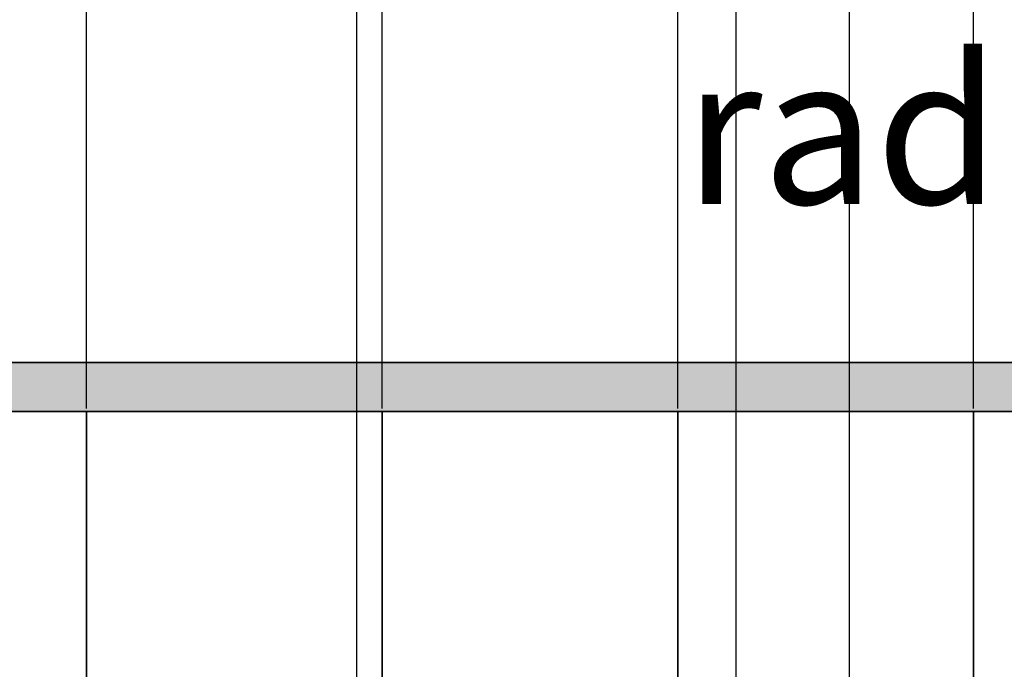
# Model space of a CAD drawing. Units: millimetres. Extents: x -22994 to 29398, y -19990 to 20176.
# Tile 31 of 135: x 119 to 139, y 43 to 56. Entities that reach past the tile are written whole.
import ezdxf

# ---------------------------------------------------------------- set-up
doc = ezdxf.new("R2010")
doc.units = ezdxf.units.MM
doc.header["$MEASUREMENT"] = 0
for name, color, linetype, lineweight in [('M-ANNO-TEXT', 7, 'Continuous', 25), ('M-DIMS', 2, 'Continuous', 18), ('M-EQPM-PATT', 7, 'Continuous', 18), ('M-PIPE', 7, 'Continuous', 35)]:
    doc.layers.add(name, color=color, linetype=linetype, lineweight=lineweight)
doc.styles.get("Standard").update_dxf_attribs({"font": 'arial.ttf'})
doc.dimstyles.get("Standard").update_dxf_attribs({"dimtxt": 0.18, "dimasz": 10000, "dimexe": 0.18, "dimexo": 0.0625, "dimgap": 0.09, "dimtad": 0, "dimtih": 1, "dimtoh": 1, "dimdec": 0, "dimzin": 0, "dimdsep": 46, "dimtxsty": 'Standard', "dimcen": 0.09, "dimadec": 0, "dimazin": 0, "dimtfac": 1, "dimtdec": 0, "dimtofl": 0, "dimtmove": 0, "dimatfit": 3, "dimfxl": 1, "dimtolj": 1, "dimtzin": 0, "dimlwd": 30, "dimarcsym": 0})

# ---------------------------------------------------------------- blocks, each defined once
blk = doc.blocks.new('*D2')
at = {"layer": 'Defpoints', "color": 0, "transparency": 16777216}
for p in [(6.677, 10.271), (290.852, 10.271), (290.852, -5.079)]:
    blk.add_point(p, dxfattribs=at)
at = {"layer": 'M-DIMS', "color": 0, "lineweight": -2, "transparency": 16777216}
for p, q in [((6.677, 10.209), (6.677, -5.259)), ((290.852, 10.209), (290.852, -5.259))]:
    blk.add_line(p, q, dxfattribs=at)
at = {"layer": 'M-DIMS', "color": 0, "lineweight": 30, "transparency": 16777216}
for p, q in [((-9993.323, -5.079), (-19993.323, -5.079)), ((10290.852, -5.079), (20290.852, -5.079))]:
    blk.add_line(p, q, dxfattribs=at)
at = {"layer": 'M-DIMS', "color": 0, "transparency": 16777216}
for points in [[(-9993.323, 1661.588), (-9993.323, -1671.745), (6.677, -5.079)], [(10290.852, 1661.588), (10290.852, -1671.745), (290.852, -5.079)]]:
    blk.add_solid(points, dxfattribs=at)
at = {"layer": 'M-DIMS', "color": 0, "transparency": 16777216, "insert": (148.765, -5.079), "char_height": 0.18, "attachment_point": 5}
blk.add_mtext('\\A1;284.2', dxfattribs=at)
blk = doc.blocks.new('*D3')
at = {"layer": 'Defpoints', "color": 0, "transparency": 16777216}
for p in [(110.265, 204.165), (110.265, 176.366), (95.833, 127.967)]:
    blk.add_point(p, dxfattribs=at)
at = {"layer": 'M-DIMS', "color": 0, "lineweight": -2, "transparency": 16777216}
for p, q in [((95.833, 128.03), (95.833, 204.345)), ((110.265, 176.429), (110.265, 204.345))]:
    blk.add_line(p, q, dxfattribs=at)
at = {"layer": 'M-DIMS', "color": 0, "lineweight": 30, "transparency": 16777216}
for p, q in [((-9904.167, 204.165), (-19904.167, 204.165)), ((10110.265, 204.165), (20110.265, 204.165))]:
    blk.add_line(p, q, dxfattribs=at)
at = {"layer": 'M-DIMS', "color": 0, "transparency": 16777216}
for points in [[(-9904.167, 1870.832), (-9904.167, -1462.501), (95.833, 204.165)], [(10110.265, 1870.832), (10110.265, -1462.501), (110.265, 204.165)]]:
    blk.add_solid(points, dxfattribs=at)
at = {"layer": 'M-DIMS', "color": 0, "transparency": 16777216, "insert": (103.049, 204.165), "char_height": 0.18, "attachment_point": 5}
blk.add_mtext('\\A1;14.432', dxfattribs=at)
blk = doc.blocks.new('*D4')
at = {"layer": 'Defpoints', "color": 0, "transparency": 16777216}
for p in [(116.265, 204.165), (110.265, 176.366), (116.265, 176.366)]:
    blk.add_point(p, dxfattribs=at)
at = {"layer": 'M-DIMS', "color": 0, "lineweight": -2, "transparency": 16777216}
for p, q in [((110.265, 176.429), (110.265, 204.345)), ((116.265, 176.429), (116.265, 204.345))]:
    blk.add_line(p, q, dxfattribs=at)
at = {"layer": 'M-DIMS', "color": 0, "lineweight": 30, "transparency": 16777216}
for p, q in [((-9889.735, 204.165), (-19889.735, 204.165)), ((10116.265, 204.165), (20116.265, 204.165))]:
    blk.add_line(p, q, dxfattribs=at)
at = {"layer": 'M-DIMS', "color": 0, "transparency": 16777216}
for points in [[(-9889.735, 1870.832), (-9889.735, -1462.501), (110.265, 204.165)], [(10116.265, 1870.832), (10116.265, -1462.501), (116.265, 204.165)]]:
    blk.add_solid(points, dxfattribs=at)
at = {"layer": 'M-DIMS', "color": 0, "transparency": 16777216, "insert": (113.265, 204.165), "char_height": 0.18, "attachment_point": 5}
blk.add_mtext('\\A1;6', dxfattribs=at)
blk = doc.blocks.new('*D5')
at = {"layer": 'Defpoints', "color": 0, "transparency": 16777216}
for p in [(181.265, 204.165), (116.265, 176.366), (181.265, 176.366)]:
    blk.add_point(p, dxfattribs=at)
at = {"layer": 'M-DIMS', "color": 0, "lineweight": -2, "transparency": 16777216}
for p, q in [((116.265, 176.429), (116.265, 204.345)), ((181.265, 176.429), (181.265, 204.345))]:
    blk.add_line(p, q, dxfattribs=at)
at = {"layer": 'M-DIMS', "color": 0, "lineweight": 30, "transparency": 16777216}
for p, q in [((-9883.735, 204.165), (-19883.735, 204.165)), ((10181.265, 204.165), (20181.265, 204.165))]:
    blk.add_line(p, q, dxfattribs=at)
at = {"layer": 'M-DIMS', "color": 0, "transparency": 16777216}
for points in [[(-9883.735, 1870.832), (-9883.735, -1462.501), (116.265, 204.165)], [(10181.265, 1870.832), (10181.265, -1462.501), (181.265, 204.165)]]:
    blk.add_solid(points, dxfattribs=at)
at = {"layer": 'M-DIMS', "color": 0, "transparency": 16777216, "insert": (148.765, 204.165), "char_height": 0.18, "attachment_point": 5}
blk.add_mtext('\\A1;65', dxfattribs=at)
blk = doc.blocks.new('*D6')
at = {"layer": 'Defpoints', "color": 0, "transparency": 16777216}
for p in [(187.265, 204.165), (181.265, 176.366), (187.265, 176.366)]:
    blk.add_point(p, dxfattribs=at)
at = {"layer": 'M-DIMS', "color": 0, "lineweight": -2, "transparency": 16777216}
for p, q in [((181.265, 176.429), (181.265, 204.345)), ((187.265, 176.429), (187.265, 204.345))]:
    blk.add_line(p, q, dxfattribs=at)
at = {"layer": 'M-DIMS', "color": 0, "lineweight": 30, "transparency": 16777216}
for p, q in [((-9818.735, 204.165), (-19818.735, 204.165)), ((10187.265, 204.165), (20187.265, 204.165))]:
    blk.add_line(p, q, dxfattribs=at)
at = {"layer": 'M-DIMS', "color": 0, "transparency": 16777216}
for points in [[(-9818.735, 1870.832), (-9818.735, -1462.501), (181.265, 204.165)], [(10187.265, 1870.832), (10187.265, -1462.501), (187.265, 204.165)]]:
    blk.add_solid(points, dxfattribs=at)
at = {"layer": 'M-DIMS', "color": 0, "transparency": 16777216, "insert": (184.265, 204.165), "char_height": 0.18, "attachment_point": 5}
blk.add_mtext('\\A1;6', dxfattribs=at)
blk = doc.blocks.new('*D7')
at = {"layer": 'Defpoints', "color": 0, "transparency": 16777216}
for p in [(201.697, 204.165), (187.265, 176.366), (201.697, 127.967)]:
    blk.add_point(p, dxfattribs=at)
at = {"layer": 'M-DIMS', "color": 0, "lineweight": -2, "transparency": 16777216}
for p, q in [((187.265, 176.429), (187.265, 204.345)), ((201.697, 128.03), (201.697, 204.345))]:
    blk.add_line(p, q, dxfattribs=at)
at = {"layer": 'M-DIMS', "color": 0, "lineweight": 30, "transparency": 16777216}
for p, q in [((-9812.735, 204.165), (-19812.735, 204.165)), ((10201.697, 204.165), (20201.697, 204.165))]:
    blk.add_line(p, q, dxfattribs=at)
at = {"layer": 'M-DIMS', "color": 0, "transparency": 16777216}
for points in [[(-9812.735, 1870.832), (-9812.735, -1462.501), (187.265, 204.165)], [(10201.697, 1870.832), (10201.697, -1462.501), (201.697, 204.165)]]:
    blk.add_solid(points, dxfattribs=at)
at = {"layer": 'M-DIMS', "color": 0, "transparency": 16777216, "insert": (194.481, 204.165), "char_height": 0.18, "attachment_point": 5}
blk.add_mtext('\\A1;14.432', dxfattribs=at)
blk = doc.blocks.new('*D8')
at = {"layer": 'Defpoints', "color": 0, "transparency": 16777216}
for p in [(227.648, 204.165), (227.648, 146.73), (201.697, 127.967)]:
    blk.add_point(p, dxfattribs=at)
at = {"layer": 'M-DIMS', "color": 0, "lineweight": -2, "transparency": 16777216}
for p, q in [((201.697, 128.03), (201.697, 204.345)), ((227.648, 146.792), (227.648, 204.345))]:
    blk.add_line(p, q, dxfattribs=at)
at = {"layer": 'M-DIMS', "color": 0, "lineweight": 30, "transparency": 16777216}
for p, q in [((-9798.303, 204.165), (-19798.303, 204.165)), ((10227.648, 204.165), (20227.648, 204.165))]:
    blk.add_line(p, q, dxfattribs=at)
at = {"layer": 'M-DIMS', "color": 0, "transparency": 16777216}
for points in [[(-9798.303, 1870.832), (-9798.303, -1462.501), (201.697, 204.165)], [(10227.648, 1870.832), (10227.648, -1462.501), (227.648, 204.165)]]:
    blk.add_solid(points, dxfattribs=at)
at = {"layer": 'M-DIMS', "color": 0, "transparency": 16777216, "insert": (214.673, 204.165), "char_height": 0.18, "attachment_point": 5}
blk.add_mtext('\\A1;25.95', dxfattribs=at)
blk = doc.blocks.new('*D9')
at = {"layer": 'Defpoints', "color": 0, "transparency": 16777216}
for p in [(187.265, 176.366), (306.202, 176.366), (290.852, 10.271)]:
    blk.add_point(p, dxfattribs=at)
at = {"layer": 'M-DIMS', "color": 0, "lineweight": 30, "transparency": 16777216}
for p, q in [((306.202, 10176.366), (306.202, 20176.366)), ((306.202, -9989.729), (306.202, -19989.729))]:
    blk.add_line(p, q, dxfattribs=at)
at = {"layer": 'M-DIMS', "color": 0, "lineweight": -2, "transparency": 16777216}
for p, q in [((187.327, 176.366), (306.382, 176.366)), ((290.915, 10.271), (306.382, 10.271))]:
    blk.add_line(p, q, dxfattribs=at)
at = {"layer": 'M-DIMS', "color": 0, "transparency": 16777216}
for points in [[(-1360.465, 10176.366), (1972.869, 10176.366), (306.202, 176.366)], [(-1360.465, -9989.729), (1972.869, -9989.729), (306.202, 10.271)]]:
    blk.add_solid(points, dxfattribs=at)
at = {"layer": 'M-DIMS', "color": 0, "transparency": 16777216, "insert": (306.202, 93.319), "char_height": 0.18, "attachment_point": 5}
blk.add_mtext('\\A1;166.1', dxfattribs=at)
blk = doc.blocks.new('*D10')
at = {"layer": 'Defpoints', "color": 0, "transparency": 16777216}
for p in [(125.65, 136.071), (133.346, 136.071), (133.346, -5.079)]:
    blk.add_point(p, dxfattribs=at)
at = {"layer": 'M-DIMS', "color": 0, "lineweight": -2, "transparency": 16777216}
for p, q in [((125.65, 136.009), (125.65, -5.259)), ((133.346, 136.009), (133.346, -5.259))]:
    blk.add_line(p, q, dxfattribs=at)
at = {"layer": 'M-DIMS', "color": 0, "lineweight": 30, "transparency": 16777216}
for p, q in [((-9874.35, -5.079), (-19874.35, -5.079)), ((10133.346, -5.079), (20133.346, -5.079))]:
    blk.add_line(p, q, dxfattribs=at)
at = {"layer": 'M-DIMS', "color": 0, "transparency": 16777216}
for points in [[(-9874.35, 1661.588), (-9874.35, -1671.745), (125.65, -5.079)], [(10133.346, 1661.588), (10133.346, -1671.745), (133.346, -5.079)]]:
    blk.add_solid(points, dxfattribs=at)
at = {"layer": 'M-DIMS', "color": 0, "transparency": 16777216, "insert": (129.498, -5.079), "char_height": 0.18, "attachment_point": 5}
blk.add_mtext('\\A1;7.696', dxfattribs=at)
blk = doc.blocks.new('*D11')
at = {"layer": 'Defpoints', "color": 0, "transparency": 16777216}
for p in [(133.346, 136.071), (135.65, 136.071), (135.65, -5.079)]:
    blk.add_point(p, dxfattribs=at)
at = {"layer": 'M-DIMS', "color": 0, "lineweight": -2, "transparency": 16777216}
for p, q in [((133.346, 136.009), (133.346, -5.259)), ((135.65, 136.009), (135.65, -5.259))]:
    blk.add_line(p, q, dxfattribs=at)
at = {"layer": 'M-DIMS', "color": 0, "lineweight": 30, "transparency": 16777216}
for p, q in [((-9866.654, -5.079), (-19866.654, -5.079)), ((10135.65, -5.079), (20135.65, -5.079))]:
    blk.add_line(p, q, dxfattribs=at)
at = {"layer": 'M-DIMS', "color": 0, "transparency": 16777216}
for points in [[(-9866.654, 1661.588), (-9866.654, -1671.745), (133.346, -5.079)], [(10135.65, 1661.588), (10135.65, -1671.745), (135.65, -5.079)]]:
    blk.add_solid(points, dxfattribs=at)
at = {"layer": 'M-DIMS', "color": 0, "transparency": 16777216, "insert": (134.498, -5.079), "char_height": 0.18, "attachment_point": 5}
blk.add_mtext('\\A1;2.304', dxfattribs=at)
blk = doc.blocks.new('*D12')
at = {"layer": 'Defpoints', "color": 0, "transparency": 16777216}
for p in [(135.65, 136.071), (145.65, 136.071), (145.65, -5.079)]:
    blk.add_point(p, dxfattribs=at)
at = {"layer": 'M-DIMS', "color": 0, "lineweight": -2, "transparency": 16777216}
for p, q in [((135.65, 136.009), (135.65, -5.259)), ((145.65, 136.009), (145.65, -5.259))]:
    blk.add_line(p, q, dxfattribs=at)
at = {"layer": 'M-DIMS', "color": 0, "lineweight": 30, "transparency": 16777216}
for p, q in [((-9864.35, -5.079), (-19864.35, -5.079)), ((10145.65, -5.079), (20145.65, -5.079))]:
    blk.add_line(p, q, dxfattribs=at)
at = {"layer": 'M-DIMS', "color": 0, "transparency": 16777216}
for points in [[(-9864.35, 1661.588), (-9864.35, -1671.745), (135.65, -5.079)], [(10145.65, 1661.588), (10145.65, -1671.745), (145.65, -5.079)]]:
    blk.add_solid(points, dxfattribs=at)
at = {"layer": 'M-DIMS', "color": 0, "transparency": 16777216, "insert": (140.65, -5.079), "char_height": 0.18, "attachment_point": 5}
blk.add_mtext('\\A1;10', dxfattribs=at)
blk = doc.blocks.new('*D13')
at = {"layer": 'Defpoints', "color": 0, "transparency": 16777216}
for p in [(145.65, 136.071), (155.65, 136.071), (155.65, -5.079)]:
    blk.add_point(p, dxfattribs=at)
at = {"layer": 'M-DIMS', "color": 0, "lineweight": -2, "transparency": 16777216}
for p, q in [((145.65, 136.009), (145.65, -5.259)), ((155.65, 136.009), (155.65, -5.259))]:
    blk.add_line(p, q, dxfattribs=at)
at = {"layer": 'M-DIMS', "color": 0, "lineweight": 30, "transparency": 16777216}
for p, q in [((-9854.35, -5.079), (-19854.35, -5.079)), ((10155.65, -5.079), (20155.65, -5.079))]:
    blk.add_line(p, q, dxfattribs=at)
at = {"layer": 'M-DIMS', "color": 0, "transparency": 16777216}
for points in [[(-9854.35, 1661.588), (-9854.35, -1671.745), (145.65, -5.079)], [(10155.65, 1661.588), (10155.65, -1671.745), (155.65, -5.079)]]:
    blk.add_solid(points, dxfattribs=at)
at = {"layer": 'M-DIMS', "color": 0, "transparency": 16777216, "insert": (150.65, -5.079), "char_height": 0.18, "attachment_point": 5}
blk.add_mtext('\\A1;10', dxfattribs=at)
blk = doc.blocks.new('*D14')
at = {"layer": 'Defpoints', "color": 0, "transparency": 16777216}
for p in [(155.65, 136.071), (165.65, 136.071), (165.65, -5.079)]:
    blk.add_point(p, dxfattribs=at)
at = {"layer": 'M-DIMS', "color": 0, "lineweight": -2, "transparency": 16777216}
for p, q in [((155.65, 136.009), (155.65, -5.259)), ((165.65, 136.009), (165.65, -5.259))]:
    blk.add_line(p, q, dxfattribs=at)
at = {"layer": 'M-DIMS', "color": 0, "lineweight": 30, "transparency": 16777216}
for p, q in [((-9844.35, -5.079), (-19844.35, -5.079)), ((10165.65, -5.079), (20165.65, -5.079))]:
    blk.add_line(p, q, dxfattribs=at)
at = {"layer": 'M-DIMS', "color": 0, "transparency": 16777216}
for points in [[(-9844.35, 1661.588), (-9844.35, -1671.745), (155.65, -5.079)], [(10165.65, 1661.588), (10165.65, -1671.745), (165.65, -5.079)]]:
    blk.add_solid(points, dxfattribs=at)
at = {"layer": 'M-DIMS', "color": 0, "transparency": 16777216, "insert": (160.65, -5.079), "char_height": 0.18, "attachment_point": 5}
blk.add_mtext('\\A1;10', dxfattribs=at)
blk = doc.blocks.new('*D15')
at = {"layer": 'Defpoints', "color": 0, "transparency": 16777216}
for p in [(173.346, 154.788), (173.346, 136.071), (306.202, 136.071)]:
    blk.add_point(p, dxfattribs=at)
at = {"layer": 'M-DIMS', "color": 0, "lineweight": 30, "transparency": 16777216}
for p, q in [((306.202, 10154.788), (306.202, 20154.788)), ((306.202, -9863.929), (306.202, -19863.929))]:
    blk.add_line(p, q, dxfattribs=at)
at = {"layer": 'M-DIMS', "color": 0, "lineweight": -2, "transparency": 16777216}
for p, q in [((173.408, 154.788), (306.382, 154.788)), ((173.408, 136.071), (306.382, 136.071))]:
    blk.add_line(p, q, dxfattribs=at)
at = {"layer": 'M-DIMS', "color": 0, "transparency": 16777216}
for points in [[(-1360.465, 10154.788), (1972.869, 10154.788), (306.202, 154.788)], [(-1360.465, -9863.929), (1972.869, -9863.929), (306.202, 136.071)]]:
    blk.add_solid(points, dxfattribs=at)
at = {"layer": 'M-DIMS', "color": 0, "transparency": 16777216, "insert": (306.202, 145.43), "char_height": 0.18, "attachment_point": 5}
blk.add_mtext('\\A1;18.717', dxfattribs=at)
blk = doc.blocks.new('*D16')
at = {"layer": 'Defpoints', "color": 0, "transparency": 16777216}
for p in [(120.17, 204.165), (110.466, 48.035), (120.17, 48.035)]:
    blk.add_point(p, dxfattribs=at)
at = {"layer": 'M-DIMS', "color": 0, "lineweight": -2, "transparency": 16777216}
for p, q in [((110.466, 48.097), (110.466, 204.345)), ((120.17, 48.097), (120.17, 204.345))]:
    blk.add_line(p, q, dxfattribs=at)
at = {"layer": 'M-DIMS', "color": 0, "lineweight": 30, "transparency": 16777216}
for p, q in [((-9889.534, 204.165), (-19889.534, 204.165)), ((10120.17, 204.165), (20120.17, 204.165))]:
    blk.add_line(p, q, dxfattribs=at)
at = {"layer": 'M-DIMS', "color": 0, "transparency": 16777216}
for points in [[(-9889.534, 1870.832), (-9889.534, -1462.501), (110.466, 204.165)], [(10120.17, 1870.832), (10120.17, -1462.501), (120.17, 204.165)]]:
    blk.add_solid(points, dxfattribs=at)
at = {"layer": 'M-DIMS', "color": 0, "transparency": 16777216, "insert": (115.318, 204.165), "char_height": 0.18, "attachment_point": 5}
blk.add_mtext('\\A1;9.704', dxfattribs=at)
blk = doc.blocks.new('*D17')
at = {"layer": 'Defpoints', "color": 0, "transparency": 16777216}
for p in [(126.17, 204.165), (120.17, 48.035), (126.17, 48.035)]:
    blk.add_point(p, dxfattribs=at)
at = {"layer": 'M-DIMS', "color": 0, "lineweight": -2, "transparency": 16777216}
for p, q in [((120.17, 48.097), (120.17, 204.345)), ((126.17, 48.097), (126.17, 204.345))]:
    blk.add_line(p, q, dxfattribs=at)
at = {"layer": 'M-DIMS', "color": 0, "lineweight": 30, "transparency": 16777216}
for p, q in [((-9879.83, 204.165), (-19879.83, 204.165)), ((10126.17, 204.165), (20126.17, 204.165))]:
    blk.add_line(p, q, dxfattribs=at)
at = {"layer": 'M-DIMS', "color": 0, "transparency": 16777216}
for points in [[(-9879.83, 1870.832), (-9879.83, -1462.501), (120.17, 204.165)], [(10126.17, 1870.832), (10126.17, -1462.501), (126.17, 204.165)]]:
    blk.add_solid(points, dxfattribs=at)
at = {"layer": 'M-DIMS', "color": 0, "transparency": 16777216, "insert": (123.17, 204.165), "char_height": 0.18, "attachment_point": 5}
blk.add_mtext('\\A1;6', dxfattribs=at)
blk = doc.blocks.new('*D18')
at = {"layer": 'Defpoints', "color": 0, "transparency": 16777216}
for p in [(132.17, 204.165), (126.17, 48.035), (132.17, 48.035)]:
    blk.add_point(p, dxfattribs=at)
at = {"layer": 'M-DIMS', "color": 0, "lineweight": -2, "transparency": 16777216}
for p, q in [((126.17, 48.097), (126.17, 204.345)), ((132.17, 48.097), (132.17, 204.345))]:
    blk.add_line(p, q, dxfattribs=at)
at = {"layer": 'M-DIMS', "color": 0, "lineweight": 30, "transparency": 16777216}
for p, q in [((-9873.83, 204.165), (-19873.83, 204.165)), ((10132.17, 204.165), (20132.17, 204.165))]:
    blk.add_line(p, q, dxfattribs=at)
at = {"layer": 'M-DIMS', "color": 0, "transparency": 16777216}
for points in [[(-9873.83, 1870.832), (-9873.83, -1462.501), (126.17, 204.165)], [(10132.17, 1870.832), (10132.17, -1462.501), (132.17, 204.165)]]:
    blk.add_solid(points, dxfattribs=at)
at = {"layer": 'M-DIMS', "color": 0, "transparency": 16777216, "insert": (129.17, 204.165), "char_height": 0.18, "attachment_point": 5}
blk.add_mtext('\\A1;6', dxfattribs=at)
blk = doc.blocks.new('*D19')
at = {"layer": 'Defpoints', "color": 0, "transparency": 16777216}
for p in [(138.17, 204.165), (132.17, 48.035), (138.17, 48.035)]:
    blk.add_point(p, dxfattribs=at)
at = {"layer": 'M-DIMS', "color": 0, "lineweight": -2, "transparency": 16777216}
for p, q in [((132.17, 48.097), (132.17, 204.345)), ((138.17, 48.097), (138.17, 204.345))]:
    blk.add_line(p, q, dxfattribs=at)
at = {"layer": 'M-DIMS', "color": 0, "lineweight": 30, "transparency": 16777216}
for p, q in [((-9867.83, 204.165), (-19867.83, 204.165)), ((10138.17, 204.165), (20138.17, 204.165))]:
    blk.add_line(p, q, dxfattribs=at)
at = {"layer": 'M-DIMS', "color": 0, "transparency": 16777216}
for points in [[(-9867.83, 1870.832), (-9867.83, -1462.501), (132.17, 204.165)], [(10138.17, 1870.832), (10138.17, -1462.501), (138.17, 204.165)]]:
    blk.add_solid(points, dxfattribs=at)
at = {"layer": 'M-DIMS', "color": 0, "transparency": 16777216, "insert": (135.17, 204.165), "char_height": 0.18, "attachment_point": 5}
blk.add_mtext('\\A1;6', dxfattribs=at)
blk = doc.blocks.new('*D20')
at = {"layer": 'Defpoints', "color": 0, "transparency": 16777216}
for p in [(144.17, 204.165), (138.17, 48.035), (144.17, 48.035)]:
    blk.add_point(p, dxfattribs=at)
at = {"layer": 'M-DIMS', "color": 0, "lineweight": -2, "transparency": 16777216}
for p, q in [((138.17, 48.097), (138.17, 204.345)), ((144.17, 48.097), (144.17, 204.345))]:
    blk.add_line(p, q, dxfattribs=at)
at = {"layer": 'M-DIMS', "color": 0, "lineweight": 30, "transparency": 16777216}
for p, q in [((-9861.83, 204.165), (-19861.83, 204.165)), ((10144.17, 204.165), (20144.17, 204.165))]:
    blk.add_line(p, q, dxfattribs=at)
at = {"layer": 'M-DIMS', "color": 0, "transparency": 16777216}
for points in [[(-9861.83, 1870.832), (-9861.83, -1462.501), (138.17, 204.165)], [(10144.17, 1870.832), (10144.17, -1462.501), (144.17, 204.165)]]:
    blk.add_solid(points, dxfattribs=at)
at = {"layer": 'M-DIMS', "color": 0, "transparency": 16777216, "insert": (141.17, 204.165), "char_height": 0.18, "attachment_point": 5}
blk.add_mtext('\\A1;6', dxfattribs=at)
blk = doc.blocks.new('*D21')
at = {"layer": 'Defpoints', "color": 0, "transparency": 16777216}
for p in [(149.116, 204.165), (144.17, 48.035), (149.116, 48.035)]:
    blk.add_point(p, dxfattribs=at)
at = {"layer": 'M-DIMS', "color": 0, "lineweight": -2, "transparency": 16777216}
for p, q in [((144.17, 48.097), (144.17, 204.345)), ((149.116, 48.097), (149.116, 204.345))]:
    blk.add_line(p, q, dxfattribs=at)
at = {"layer": 'M-DIMS', "color": 0, "lineweight": 30, "transparency": 16777216}
for p, q in [((-9855.83, 204.165), (-19855.83, 204.165)), ((10149.116, 204.165), (20149.116, 204.165))]:
    blk.add_line(p, q, dxfattribs=at)
at = {"layer": 'M-DIMS', "color": 0, "transparency": 16777216}
for points in [[(-9855.83, 1870.832), (-9855.83, -1462.501), (144.17, 204.165)], [(10149.116, 1870.832), (10149.116, -1462.501), (149.116, 204.165)]]:
    blk.add_solid(points, dxfattribs=at)
at = {"layer": 'M-DIMS', "color": 0, "transparency": 16777216, "insert": (146.643, 204.165), "char_height": 0.18, "attachment_point": 5}
blk.add_mtext('\\A1;4.945', dxfattribs=at)
blk = doc.blocks.new('*D22')
at = {"layer": 'Defpoints', "color": 0, "transparency": 16777216}
for p in [(149.116, 30.99), (155.116, 30.99), (155.116, -5.079)]:
    blk.add_point(p, dxfattribs=at)
at = {"layer": 'M-DIMS', "color": 0, "lineweight": -2, "transparency": 16777216}
for p, q in [((149.116, 30.927), (149.116, -5.259)), ((155.116, 30.927), (155.116, -5.259))]:
    blk.add_line(p, q, dxfattribs=at)
at = {"layer": 'M-DIMS', "color": 0, "lineweight": 30, "transparency": 16777216}
for p, q in [((-9850.884, -5.079), (-19850.884, -5.079)), ((10155.116, -5.079), (20155.116, -5.079))]:
    blk.add_line(p, q, dxfattribs=at)
at = {"layer": 'M-DIMS', "color": 0, "transparency": 16777216}
for points in [[(-9850.884, 1661.588), (-9850.884, -1671.745), (149.116, -5.079)], [(10155.116, 1661.588), (10155.116, -1671.745), (155.116, -5.079)]]:
    blk.add_solid(points, dxfattribs=at)
at = {"layer": 'M-DIMS', "color": 0, "transparency": 16777216, "insert": (152.116, -5.079), "char_height": 0.18, "attachment_point": 5}
blk.add_mtext('\\A1;6', dxfattribs=at)
blk = doc.blocks.new('*D23')
at = {"layer": 'Defpoints', "color": 0, "transparency": 16777216}
for p in [(155.116, 30.99), (161.116, 30.99), (161.116, -5.079)]:
    blk.add_point(p, dxfattribs=at)
at = {"layer": 'M-DIMS', "color": 0, "lineweight": -2, "transparency": 16777216}
for p, q in [((155.116, 30.927), (155.116, -5.259)), ((161.116, 30.927), (161.116, -5.259))]:
    blk.add_line(p, q, dxfattribs=at)
at = {"layer": 'M-DIMS', "color": 0, "lineweight": 30, "transparency": 16777216}
for p, q in [((-9844.884, -5.079), (-19844.884, -5.079)), ((10161.116, -5.079), (20161.116, -5.079))]:
    blk.add_line(p, q, dxfattribs=at)
at = {"layer": 'M-DIMS', "color": 0, "transparency": 16777216}
for points in [[(-9844.884, 1661.588), (-9844.884, -1671.745), (155.116, -5.079)], [(10161.116, 1661.588), (10161.116, -1671.745), (161.116, -5.079)]]:
    blk.add_solid(points, dxfattribs=at)
at = {"layer": 'M-DIMS', "color": 0, "transparency": 16777216, "insert": (158.116, -5.079), "char_height": 0.18, "attachment_point": 5}
blk.add_mtext('\\A1;6', dxfattribs=at)
blk = doc.blocks.new('*D24')
at = {"layer": 'Defpoints', "color": 0, "transparency": 16777216}
for p in [(161.116, 30.99), (166.439, 30.99), (166.439, -5.079)]:
    blk.add_point(p, dxfattribs=at)
at = {"layer": 'M-DIMS', "color": 0, "lineweight": -2, "transparency": 16777216}
for p, q in [((161.116, 30.927), (161.116, -5.259)), ((166.439, 30.927), (166.439, -5.259))]:
    blk.add_line(p, q, dxfattribs=at)
at = {"layer": 'M-DIMS', "color": 0, "lineweight": 30, "transparency": 16777216}
for p, q in [((-9838.884, -5.079), (-19838.884, -5.079)), ((10166.439, -5.079), (20166.439, -5.079))]:
    blk.add_line(p, q, dxfattribs=at)
at = {"layer": 'M-DIMS', "color": 0, "transparency": 16777216}
for points in [[(-9838.884, 1661.588), (-9838.884, -1671.745), (161.116, -5.079)], [(10166.439, 1661.588), (10166.439, -1671.745), (166.439, -5.079)]]:
    blk.add_solid(points, dxfattribs=at)
at = {"layer": 'M-DIMS', "color": 0, "transparency": 16777216, "insert": (163.777, -5.079), "char_height": 0.18, "attachment_point": 5}
blk.add_mtext('\\A1;5.323', dxfattribs=at)
blk = doc.blocks.new('*D25')
at = {"layer": 'Defpoints', "color": 0, "transparency": 16777216}
for p in [(166.439, 30.99), (172.439, 30.99), (172.439, -5.079)]:
    blk.add_point(p, dxfattribs=at)
at = {"layer": 'M-DIMS', "color": 0, "lineweight": -2, "transparency": 16777216}
for p, q in [((166.439, 30.927), (166.439, -5.259)), ((172.439, 30.927), (172.439, -5.259))]:
    blk.add_line(p, q, dxfattribs=at)
at = {"layer": 'M-DIMS', "color": 0, "lineweight": 30, "transparency": 16777216}
for p, q in [((-9833.561, -5.079), (-19833.561, -5.079)), ((10172.439, -5.079), (20172.439, -5.079))]:
    blk.add_line(p, q, dxfattribs=at)
at = {"layer": 'M-DIMS', "color": 0, "transparency": 16777216}
for points in [[(-9833.561, 1661.588), (-9833.561, -1671.745), (166.439, -5.079)], [(10172.439, 1661.588), (10172.439, -1671.745), (172.439, -5.079)]]:
    blk.add_solid(points, dxfattribs=at)
at = {"layer": 'M-DIMS', "color": 0, "transparency": 16777216, "insert": (169.439, -5.079), "char_height": 0.18, "attachment_point": 5}
blk.add_mtext('\\A1;6', dxfattribs=at)
blk = doc.blocks.new('*D26')
at = {"layer": 'Defpoints', "color": 0, "transparency": 16777216}
for p in [(172.439, 30.99), (178.439, 30.99), (178.439, -5.079)]:
    blk.add_point(p, dxfattribs=at)
at = {"layer": 'M-DIMS', "color": 0, "lineweight": -2, "transparency": 16777216}
for p, q in [((172.439, 30.927), (172.439, -5.259)), ((178.439, 30.927), (178.439, -5.259))]:
    blk.add_line(p, q, dxfattribs=at)
at = {"layer": 'M-DIMS', "color": 0, "lineweight": 30, "transparency": 16777216}
for p, q in [((-9827.561, -5.079), (-19827.561, -5.079)), ((10178.439, -5.079), (20178.439, -5.079))]:
    blk.add_line(p, q, dxfattribs=at)
at = {"layer": 'M-DIMS', "color": 0, "transparency": 16777216}
for points in [[(-9827.561, 1661.588), (-9827.561, -1671.745), (172.439, -5.079)], [(10178.439, 1661.588), (10178.439, -1671.745), (178.439, -5.079)]]:
    blk.add_solid(points, dxfattribs=at)
at = {"layer": 'M-DIMS', "color": 0, "transparency": 16777216, "insert": (175.439, -5.079), "char_height": 0.18, "attachment_point": 5}
blk.add_mtext('\\A1;6', dxfattribs=at)
blk = doc.blocks.new('*D27')
at = {"layer": 'Defpoints', "color": 0, "transparency": 16777216}
for p in [(178.439, 30.99), (188.117, 30.99), (188.117, -5.079)]:
    blk.add_point(p, dxfattribs=at)
at = {"layer": 'M-DIMS', "color": 0, "lineweight": -2, "transparency": 16777216}
for p, q in [((178.439, 30.927), (178.439, -5.259)), ((188.117, 30.927), (188.117, -5.259))]:
    blk.add_line(p, q, dxfattribs=at)
at = {"layer": 'M-DIMS', "color": 0, "lineweight": 30, "transparency": 16777216}
for p, q in [((-9821.561, -5.079), (-19821.561, -5.079)), ((10188.117, -5.079), (20188.117, -5.079))]:
    blk.add_line(p, q, dxfattribs=at)
at = {"layer": 'M-DIMS', "color": 0, "transparency": 16777216}
for points in [[(-9821.561, 1661.588), (-9821.561, -1671.745), (178.439, -5.079)], [(10188.117, 1661.588), (10188.117, -1671.745), (188.117, -5.079)]]:
    blk.add_solid(points, dxfattribs=at)
at = {"layer": 'M-DIMS', "color": 0, "transparency": 16777216, "insert": (183.278, -5.079), "char_height": 0.18, "attachment_point": 5}
blk.add_mtext('\\A1;9.679', dxfattribs=at)
blk = doc.blocks.new('*D28')
at = {"layer": 'Defpoints', "color": 0, "transparency": 16777216}
for p in [(188.117, 48.035), (306.202, 48.035), (188.117, 30.99)]:
    blk.add_point(p, dxfattribs=at)
at = {"layer": 'M-DIMS', "color": 0, "lineweight": 30, "transparency": 16777216}
for p, q in [((306.202, 10048.035), (306.202, 20048.035)), ((306.202, -9969.01), (306.202, -19969.01))]:
    blk.add_line(p, q, dxfattribs=at)
at = {"layer": 'M-DIMS', "color": 0, "lineweight": -2, "transparency": 16777216}
for p, q in [((188.18, 48.035), (306.382, 48.035)), ((188.18, 30.99), (306.382, 30.99))]:
    blk.add_line(p, q, dxfattribs=at)
at = {"layer": 'M-DIMS', "color": 0, "transparency": 16777216}
for points in [[(-1360.465, 10048.035), (1972.869, 10048.035), (306.202, 48.035)], [(-1360.465, -9969.01), (1972.869, -9969.01), (306.202, 30.99)]]:
    blk.add_solid(points, dxfattribs=at)
at = {"layer": 'M-DIMS', "color": 0, "transparency": 16777216, "insert": (306.202, 39.512), "char_height": 0.18, "attachment_point": 5}
blk.add_mtext('\\A1;17.045', dxfattribs=at)
blk = doc.blocks.new('*D29')
at = {"layer": 'Defpoints', "color": 0, "transparency": 16777216}
for p in [(36.801, 80.045), (64.03, 80.045)]:
    blk.add_point(p, dxfattribs=at)
at = {"layer": 'M-DIMS', "color": 0, "lineweight": -2, "transparency": 16777216}
for p, q in [((50.415, 79.955), (50.415, 80.135)), ((50.325, 80.045), (50.505, 80.045))]:
    blk.add_line(p, q, dxfattribs=at)
at = {"layer": 'M-DIMS', "color": 0, "lineweight": 30, "transparency": 16777216}
blk.add_line((20064.03, 80.03), (10064.03, 80.038), dxfattribs=at)
at = {"layer": 'M-DIMS', "color": 0, "transparency": 16777216}
blk.add_solid([(10064.031, 1746.704), (10064.028, -1586.629), (64.03, 80.045)], dxfattribs=at)
at = {"layer": 'M-DIMS', "color": 0, "transparency": 16777216, "insert": (20064.521, 80.03), "char_height": 0.18, "attachment_point": 5}
blk.add_mtext('\\A1;∅27.23', dxfattribs=at)
blk = doc.blocks.new('*D36')
at = {"layer": 'Defpoints', "color": 0, "transparency": 16777216}
for p in [(46.39, 31.303), (46.387, 26.593)]:
    blk.add_point(p, dxfattribs=at)
at = {"layer": 'M-DIMS', "color": 0, "lineweight": 30, "transparency": 16777216}
for p, q in [((57.15, 20031.301), (51.77, 10031.302)), ((10057.15, 20031.301), (57.15, 20031.301))]:
    blk.add_line(p, q, dxfattribs=at)
at = {"layer": 'M-DIMS', "color": 0, "lineweight": -2, "transparency": 16777216}
for p, q in [((46.389, 28.858), (46.389, 29.038)), ((46.299, 28.948), (46.479, 28.948))]:
    blk.add_line(p, q, dxfattribs=at)
at = {"layer": 'M-DIMS', "color": 0, "transparency": 16777216}
blk.add_solid([(-1614.896, 10032.199), (1718.436, 10030.405), (46.39, 31.303)], dxfattribs=at)
at = {"layer": 'M-DIMS', "color": 0, "transparency": 16777216, "insert": (10057.554, 20031.301), "char_height": 0.18, "attachment_point": 5}
blk.add_mtext('\\A1;∅4.71', dxfattribs=at)
blk = doc.blocks.new('*D37')
at = {"layer": 'Defpoints', "color": 0, "transparency": 16777216}
for p in [(54.834, 118.615), (59.494, 118.614)]:
    blk.add_point(p, dxfattribs=at)
at = {"layer": 'M-DIMS', "color": 0, "lineweight": -2, "transparency": 16777216}
for p, q in [((57.164, 118.524), (57.164, 118.704)), ((57.074, 118.614), (57.254, 118.614))]:
    blk.add_line(p, q, dxfattribs=at)
at = {"layer": 'M-DIMS', "color": 0, "lineweight": 30, "transparency": 16777216}
blk.add_line((20059.493, 116.253), (10059.494, 117.434), dxfattribs=at)
at = {"layer": 'M-DIMS', "color": 0, "transparency": 16777216}
blk.add_solid([(10059.69, 1784.1), (10059.297, -1549.233), (59.494, 118.614)], dxfattribs=at)
at = {"layer": 'M-DIMS', "color": 0, "transparency": 16777216, "insert": (20059.985, 116.253), "char_height": 0.18, "attachment_point": 5}
blk.add_mtext('\\A1;∅4.659', dxfattribs=at)

msp = doc.modelspace()

# ---------------------------------------------------------------- hatches: boundary and pattern name
at = {"layer": 'M-EQPM-PATT'}
h = msp.add_hatch(color=256, dxfattribs=at)
h.set_gradient(color1=(19, 155, 72), color2=(88, 186, 72), tint=1, name='CYLINDER')
h.paths.add_polyline_path([(109.4658, 29.9895), (189.1175, 29.9895), (189.1175, 77.6953), (128.1172, 77.6953, 0.4142136), (126.1172, 75.6953), (126.1172, 73.6953, 0.4142136), (128.1172, 71.6953), (178.5136, 71.6953, -0.4142136), (179.5136, 70.6953), (179.5136, 68.6953, -0.4142136), (178.5136, 67.6953), (128.1172, 67.6953, 0.4142136), (126.1172, 65.6953), (126.1172, 63.6953, 0.4142136), (128.1172, 61.6953), (178.5136, 61.6953, -0.4142136), (179.5136, 60.6953), (179.5136, 58.6953, -0.4142136), (178.5136, 57.6953), (109.7466, 57.6953, -0.4142136), (108.7466, 58.6953), (108.7466, 75.5922, 0.4142136), (106.7466, 77.5922), (101.8327, 77.5922), (101.8327, 76.5922), (106.7466, 76.5922, -0.4142136), (107.7466, 75.5922), (107.7466, 58.6953, 0.4142136), (109.7466, 56.6953), (178.5136, 56.6953, 0.4142136), (180.5136, 58.6953), (180.5136, 60.6953, 0.4142136), (178.5136, 62.6953), (128.1172, 62.6953, -0.4142136), (127.1172, 63.6953), (127.1172, 65.6953, -0.4142136), (128.1172, 66.6953), (178.5136, 66.6953, 0.4142136), (180.5136, 68.6953), (180.5136, 70.6953, 0.4142136), (178.5136, 72.6953), (128.1172, 72.6953, -0.4142136), (127.1172, 73.6953), (127.1172, 75.6953, -0.4142136), (128.1172, 76.6953), (188.1175, 76.6953), (188.1175, 49.0349), (110.4658, 49.0349), (110.4658, 51.9576), (101.8327, 51.9576), (101.8327, 50.9576), (109.4658, 50.9576), (109.4658, 48.5349)])
h.paths.add_polyline_path([(110.4658, 48.0349), (188.1175, 48.0349), (188.1175, 30.9895), (110.4658, 30.9895)], flags=16)
h.paths.add_polyline_path([(136.1519, 78.0082), (161.2406, 78.0082), (161.2406, 84.1903), (136.1519, 84.1903)], flags=9)

# ---------------------------------------------------------------- linework, layer by layer
at = {"layer": 'M-PIPE'}
for p, q in [((120.1702, 48.0349), (120.1702, 30.9895)), ((126.1702, 48.0349), (126.1702, 30.9895)), ((126.1702, 48.0349), (126.1702, 30.9895)), ((132.1702, 48.0349), (132.1702, 30.9895)), ((132.1702, 48.0349), (132.1702, 30.9895)), ((132.1702, 48.0349), (132.1702, 30.9895)), ((138.1702, 48.0349), (138.1702, 30.9895)), ((138.1702, 48.0349), (138.1702, 30.9895))]:
    msp.add_line(p, q, dxfattribs=at)
for points in [[(110.4658, 49.0349), (188.1175, 49.0349)], [(188.1175, 30.9895), (110.4658, 30.9895), (110.4658, 48.0349), (188.1175, 48.0349)]]:
    msp.add_lwpolyline(points, dxfattribs=at)

# ---------------------------------------------------------------- texts
at = {"layer": 'M-ANNO-TEXT', "insert": (132.2925, 55.25), "char_height": 3, "attachment_point": 1}
msp.add_mtext_dynamic_manual_height_columns('radiant evaporator', width=37.883315, gutter_width=1, heights=[0], dxfattribs=at)

# ---------------------------------------------------------------- dimensions: what is measured, and where the dimension line sits
at = {"layer": 'M-DIMS'}
for base, p1, p2, override, picture, middle in [((306.202, 176.3662), (290.852, 10.2713), (187.2647, 176.3662), {"dimdec": 1, "dimlfac": 1, "dimrnd": 0, "dimzin": 0, "dimdsep": 46, "dimlunit": 2}, '*D9', (306.202, 93.3187)), ((306.202, 136.0713), (173.3459, 154.788), (173.3459, 136.0713), {"dimdec": 3, "dimlfac": 1, "dimrnd": 0, "dimzin": 0, "dimdsep": 46, "dimlunit": 2}, '*D15', (306.202, 145.4297)), ((306.202, 48.0349), (188.1175, 30.9895), (188.1175, 48.0349), {"dimdec": 3, "dimlfac": 1, "dimrnd": 0, "dimzin": 0, "dimdsep": 46, "dimlunit": 2}, '*D28', (306.202, 39.5122))]:
    dim = msp.add_linear_dim(base=base, p1=p1, p2=p2, angle=90, dimstyle='Standard', override=override, dxfattribs=at)
    dim.commit()
    dim.dimension.update_dxf_attribs({"geometry": picture, "text_midpoint": middle})
dim = msp.add_diameter_dim_2p(p1=(46.3875, 26.5934), p2=(46.39, 31.3035), dimstyle='Standard', override={"dimdec": 2, "dimlfac": 1, "dimrnd": 0, "dimzin": 0, "dimdsep": 46, "dimlunit": 2}, dxfattribs=at)
dim.commit()
dim.dimension.update_dxf_attribs({"geometry": '*D36', "text_midpoint": (10057.5542, 20031.3006), "dimtype": 163})
for base, p1, p2, override, picture, middle in [((110.2647, 204.1654), (95.8327, 127.967), (110.2647, 176.3662), {"dimdec": 3, "dimlfac": 1, "dimrnd": 0, "dimzin": 0, "dimdsep": 46, "dimlunit": 2}, '*D3', (103.0487, 204.1654)), ((116.2647, 204.1654), (110.2647, 176.3662), (116.2647, 176.3662), {"dimdec": 0, "dimlfac": 1, "dimrnd": 0, "dimzin": 0, "dimdsep": 46, "dimlunit": 2}, '*D4', (113.2647, 204.1654)), ((120.1702, 204.1654), (110.4658, 48.0349), (120.1702, 48.0349), {"dimdec": 3, "dimlfac": 1, "dimrnd": 0, "dimzin": 0, "dimdsep": 46, "dimlunit": 2}, '*D16', (115.318, 204.1654)), ((181.2647, 204.1654), (116.2647, 176.3662), (181.2647, 176.3662), {"dimdec": 0, "dimlfac": 1, "dimrnd": 0, "dimzin": 0, "dimdsep": 46, "dimlunit": 2}, '*D5', (148.7647, 204.1654)), ((126.1702, 204.1654), (120.1702, 48.0349), (126.1702, 48.0349), {"dimdec": 0, "dimlfac": 1, "dimrnd": 0, "dimzin": 0, "dimdsep": 46, "dimlunit": 2}, '*D17', (123.1702, 204.1654)), ((132.1702, 204.1654), (126.1702, 48.0349), (132.1702, 48.0349), {"dimdec": 0, "dimlfac": 1, "dimrnd": 0, "dimzin": 0, "dimdsep": 46, "dimlunit": 2}, '*D18', (129.1702, 204.1654)), ((138.1702, 204.1654), (132.1702, 48.0349), (138.1702, 48.0349), {"dimdec": 0, "dimlfac": 1, "dimrnd": 0, "dimzin": 0, "dimdsep": 46, "dimlunit": 2}, '*D19', (135.1702, 204.1654)), ((144.1702, 204.1654), (138.1702, 48.0349), (144.1702, 48.0349), {"dimdec": 0, "dimlfac": 1, "dimrnd": 0, "dimzin": 0, "dimdsep": 46, "dimlunit": 2}, '*D20', (141.1702, 204.1654)), ((149.11567, 204.16539), (144.17023, 48.03494), (149.11567, 48.03494), {"dimdec": 3, "dimlfac": 1, "dimrnd": 0, "dimzin": 0, "dimdsep": 46, "dimlunit": 2}, '*D21', (146.64295, 204.16539)), ((187.2647, 204.1654), (181.2647, 176.3662), (187.2647, 176.3662), {"dimdec": 0, "dimlfac": 1, "dimrnd": 0, "dimzin": 0, "dimdsep": 46, "dimlunit": 2}, '*D6', (184.2647, 204.1654)), ((201.6967, 204.1654), (187.2647, 176.3662), (201.6967, 127.967), {"dimdec": 3, "dimlfac": 1, "dimrnd": 0, "dimzin": 0, "dimdsep": 46, "dimlunit": 2}, '*D7', (194.4807, 204.1654)), ((227.6485, 204.1654), (201.6967, 127.967), (227.6485, 146.7296), {"dimdec": 2, "dimlfac": 1, "dimrnd": 0, "dimzin": 0, "dimdsep": 46, "dimlunit": 2}, '*D8', (214.6726, 204.1654)), ((290.852, -5.0787), (6.6773, 10.2713), (290.852, 10.2713), {"dimdec": 1, "dimlfac": 1, "dimrnd": 0, "dimzin": 0, "dimdsep": 46, "dimlunit": 2}, '*D2', (148.7647, -5.0787)), ((133.3459, -5.0787), (125.6498, 136.0713), (133.3459, 136.0713), {"dimdec": 3, "dimlfac": 1, "dimrnd": 0, "dimzin": 0, "dimdsep": 46, "dimlunit": 2}, '*D10', (129.4978, -5.0787)), ((135.6498, -5.0787), (133.3459, 136.0713), (135.6498, 136.0713), {"dimdec": 3, "dimlfac": 1, "dimrnd": 0, "dimzin": 0, "dimdsep": 46, "dimlunit": 2}, '*D11', (134.4978, -5.0787)), ((145.6498, -5.0787), (135.6498, 136.0713), (145.6498, 136.0713), {"dimdec": 0, "dimlfac": 1, "dimrnd": 0, "dimzin": 0, "dimdsep": 46, "dimlunit": 2}, '*D12', (140.6498, -5.0787)), ((155.6498, -5.0787), (145.6498, 136.0713), (155.6498, 136.0713), {"dimdec": 0, "dimlfac": 1, "dimrnd": 0, "dimzin": 0, "dimdsep": 46, "dimlunit": 2}, '*D13', (150.6498, -5.0787)), ((155.1157, -5.0787), (149.1157, 30.9895), (155.1157, 30.9895), {"dimdec": 0, "dimlfac": 1, "dimrnd": 0, "dimzin": 0, "dimdsep": 46, "dimlunit": 2}, '*D22', (152.1157, -5.0787)), ((161.1157, -5.0787), (155.1157, 30.9895), (161.1157, 30.9895), {"dimdec": 0, "dimlfac": 1, "dimrnd": 0, "dimzin": 0, "dimdsep": 46, "dimlunit": 2}, '*D23', (158.1157, -5.0787)), ((165.6498, -5.0787), (155.6498, 136.0713), (165.6498, 136.0713), {"dimdec": 0, "dimlfac": 1, "dimrnd": 0, "dimzin": 0, "dimdsep": 46, "dimlunit": 2}, '*D14', (160.6498, -5.0787)), ((166.4387, -5.0787), (161.1157, 30.9895), (166.4387, 30.9895), {"dimdec": 3, "dimlfac": 1, "dimrnd": 0, "dimzin": 0, "dimdsep": 46, "dimlunit": 2}, '*D24', (163.7772, -5.0787)), ((172.4387, -5.0787), (166.4387, 30.9895), (172.4387, 30.9895), {"dimdec": 0, "dimlfac": 1, "dimrnd": 0, "dimzin": 0, "dimdsep": 46, "dimlunit": 2}, '*D25', (169.4387, -5.0787)), ((178.4387, -5.0787), (172.4387, 30.9895), (178.4387, 30.9895), {"dimdec": 0, "dimlfac": 1, "dimrnd": 0, "dimzin": 0, "dimdsep": 46, "dimlunit": 2}, '*D26', (175.4387, -5.0787)), ((188.1175, -5.0787), (178.4387, 30.9895), (188.1175, 30.9895), {"dimdec": 3, "dimlfac": 1, "dimrnd": 0, "dimzin": 0, "dimdsep": 46, "dimlunit": 2}, '*D27', (183.2781, -5.0787))]:
    dim = msp.add_linear_dim(base=base, p1=p1, p2=p2, dimstyle='Standard', override=override, dxfattribs=at)
    dim.commit()
    dim.dimension.update_dxf_attribs({"geometry": picture, "text_midpoint": middle})
for p1, p2, override, picture, middle in [((54.8343, 118.6145), (59.4936, 118.614), {"dimdec": 3, "dimlfac": 1, "dimrnd": 0, "dimzin": 0, "dimdsep": 46, "dimlunit": 2}, '*D37', (20059.4934, 116.2531)), ((36.8006, 80.045), (64.0296, 80.045), {"dimdec": 2, "dimlfac": 1, "dimrnd": 0, "dimzin": 0, "dimdsep": 46, "dimlunit": 2}, '*D29', (20064.0296, 80.0303))]:
    dim = msp.add_diameter_dim_2p(p1=p1, p2=p2, dimstyle='Standard', override=override, dxfattribs=at)
    dim.commit()
    dim.dimension.update_dxf_attribs({"geometry": picture, "text_midpoint": middle})

doc.saveas('drawing.dxf')
